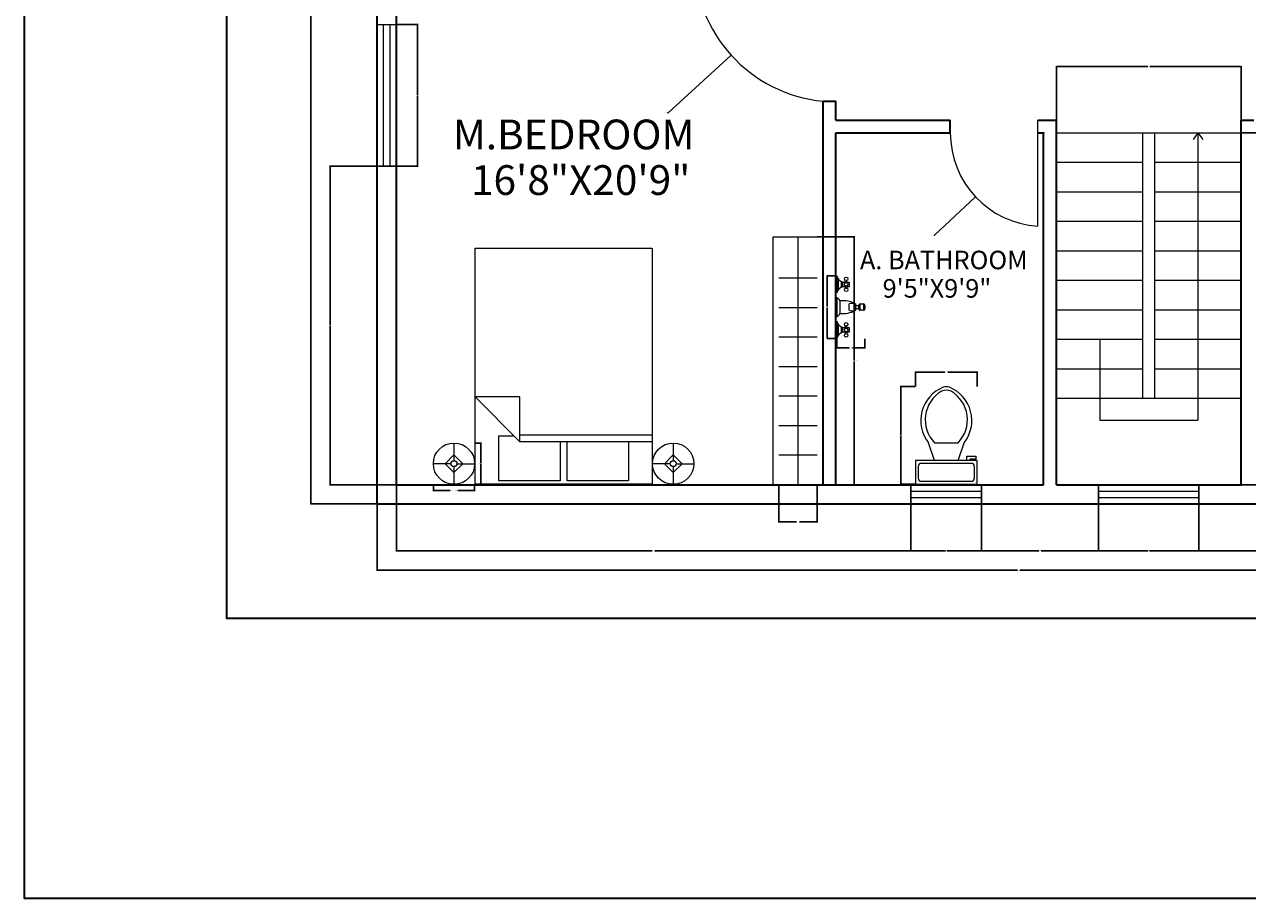
# Model space of a CAD drawing. Units: inches. Extents: x 2286 to 3750, y 1240 to 2345.
# Tile 1 of 7: x 2286 to 2701, y 1240 to 1537. Entities that reach past the tile are written whole.
import ezdxf

# ---------------------------------------------------------------- set-up
doc = ezdxf.new("R2010")
doc.units = ezdxf.units.IN
for name, color, linetype, lineweight in [('A-ANNO-DIMS', 2, 'Continuous', 18), ('A-AREA-IDEN', 7, 'Continuous', 18), ('A-DOOR', 4, 'Continuous', 18), ('A-FLOR-CASE', 8, 'Continuous', 18), ('A-FLOR-FIXT', 9, 'Continuous', 18), ('A-FLOR-STRS', 7, 'Continuous', 18), ('A-FURN', 8, 'Continuous', 18), ('A-GLAZ', 51, 'Continuous', 18), ('A-WALL', 7, 'Continuous', 35)]:
    doc.layers.add(name, color=color, linetype=linetype, lineweight=lineweight)
doc.styles.get("Standard").update_dxf_attribs({"font": 'arial.ttf'})
doc.dimstyles.get("Standard").update_dxf_attribs({"dimtxt": 0.18, "dimasz": 0.18, "dimexe": 0.18, "dimexo": 0.0625, "dimgap": 0.09, "dimtad": 0, "dimtih": 1, "dimtoh": 1, "dimdec": 4, "dimzin": 0, "dimdsep": 46, "dimtxsty": 'Standard', "dimcen": 0.09, "dimadec": 0, "dimazin": 0, "dimtfac": 1, "dimtdec": 4, "dimtofl": 0, "dimtmove": 0, "dimatfit": 3, "dimfxl": 1, "dimtolj": 1, "dimtzin": 0, "dimarcsym": 0})

# ---------------------------------------------------------------- blocks, each defined once
blk = doc.blocks.new('Faucet - Bathroom front')
for p, q in [((-0.5, 4.25), (0.5, 4.25)), ((0.5, 3.75), (-0.5, 3.75)), ((-0.5, 3), (0.5, 3)), ((0.5, 2), (-0.5, 2)), ((-0.25, 3), (-0.25, 3.5)), ((0.25, 3.5), (0.25, 3)), ((-5, 0), (-2.25, 0)), ((-4.5087, 0.25), (-2.7408, 0.25)), ((-4, 1.625), (-4.25, 1.625)), ((-4, 1.375), (-4.25, 1.375)), ((-3.1442, 0.75), (-4.0979, 0.75)), ((-3.25, 1.625), (-3, 1.625)), ((-3.25, 1.375), (-3, 1.375)), ((-1.5, 0), (1.5, 0)), ((-1, 0.5), (1, 0.5)), ((2.25, 0), (5, 0)), ((2.7413, 0.25), (4.5092, 0.25)), ((3.25, 1.625), (3, 1.625)), ((3.25, 1.375), (3, 1.375)), ((4.1058, 0.75), (3.1521, 0.75)), ((4, 1.625), (4.25, 1.625)), ((4, 1.375), (4.25, 1.375))]:
    blk.add_line(p, q)
for points in [[(-0.5, 3.75), (-0.5, 4.25)], [(-0.25, 4.5), (0.25, 4.5)], [(0.5, 4.25), (0.5, 3.75)], [(0.25, 3.5), (-0.25, 3.5)]]:
    blk.add_lwpolyline(points)
for points in [[(-4, 1), (-4, 2), (-3.25, 2), (-3.25, 1)], [(3.25, 1), (3.25, 2), (4, 2), (4, 1)]]:
    blk.add_lwpolyline(points, close=True)
for centre in [(-4.5, 1.5), (-3.625, 1.5), (-2.75, 1.5), (2.75, 1.5), (3.625, 1.5), (4.5, 1.5)]:
    blk.add_circle(centre, 0.2795)
for centre, radius, start, end in [((-0.2575, 4.2575), 0.2426, 88.22243, 181.7776), ((0.2575, 4.2575), 0.2426, 358.2224, 91.77757), ((3, 1), 4.0311, 150.2551, 187.125), ((0.6413, 2.5), 1.246, 156.3417, 203.6583), ((-0.2575, 3.7425), 0.2426, 178.2224, 271.7776), ((0.2575, 3.7425), 0.2426, 268.2224, 1.777565), ((-3, 1), 4.0311, 352.875, 29.74488), ((-0.6413, 2.5), 1.246, 336.3417, 23.65835), ((-5.375, 1.375), 1.4252, 285.2551, 344.7449), ((-1.875, 1.375), 1.4252, 195.2551, 254.7449), ((-0.7962, -0.2038), 0.7327, 106.1502, 163.8498), ((0.7962, -0.2038), 0.7327, 16.1502, 73.84979), ((1.875, 1.375), 1.4252, 285.2551, 344.7449), ((5.375, 1.375), 1.4252, 195.2551, 254.7449)]:
    blk.add_arc(centre, radius, start, end)
blk = doc.blocks.new('Bed - Queen')
for p, q in [((0, -80.00003), (0, 0)), ((0, 0), (59.99999, 0)), ((59.99999, 0), (59.99999, -80.00003)), ((7.99999, -1.2), (28.79998, -1.2)), ((7.99999, -14.4), (7.99999, -1.2)), ((28.79998, -1.2), (28.79998, -14.4)), ((31.19999, -1.2), (51.99999, -1.2)), ((31.19999, -14.4), (31.19999, -1.2)), ((51.99999, -1.2), (51.99999, -16.4)), ((0, -14.4), (44.8, -14.4)), ((59.99999, -29.6), (44.8, -14.4)), ((44.8, -14.4), (44.8, -29.6)), ((51.99999, -16.4), (46.79936, -16.4)), ((44.8, -16.8), (0, -16.8)), ((44.8, -29.6), (59.99999, -29.6)), ((59.99999, -80.00003), (0, -80.00003))]:
    blk.add_line(p, q)
blk = doc.blocks.new('Lamp - Table')
for p, q in [((0, 7), (0, 1)), ((-1, 0), (-7, 0)), ((0, 3), (-3, 0)), ((-3, 0), (0, -3)), ((3, 0), (0, 3)), ((0, -3), (3, 0)), ((1, 0), (7, 0)), ((0, -1), (0, -7))]:
    blk.add_line(p, q)
for radius in [7, 1]:
    blk.add_circle((0, 0), radius)
blk = doc.blocks.new('Toilet - top')
for p, q in [((9.5, -6), (9.5, -2)), ((-8, -8.5), (-8, -8)), ((-7, -8), (-7, -9.5)), ((-4, -8), (-6, -14)), ((4, -8), (6, -14)), ((-10, -8.5), (-8, -8.5)), ((-10, -9.5), (-10, -8.5)), ((-7, -9.5), (-10, -9.5)), ((4, -14), (-4, -14))]:
    blk.add_line(p, q)
blk.add_lwpolyline([(10.5, -8), (10.5, 0), (-10.5, 0), (-10.5, -8)], close=True)
for points in [[(-9.5, -2), (-9.5, -6)], [(8.5, -1), (-8.5, -1)], [(-8.5, -7), (8.5, -7)]]:
    blk.add_lwpolyline(points)
for centre, radius, start, end in [((-8.62, -1.88), 0.884, 81.8699, 188.1301), ((8.62, -1.88), 0.884, 351.8699, 98.1301), ((-8.62, -6.12), 0.884, 171.8699, 278.1301), ((8.62, -6.12), 0.884, 261.8699, 8.1301), ((3.52, -21.58), 12.17, 141.4691, 247.9714), ((4.2, -21.82), 11.33, 136.3677, 238.9468), ((-3.52, -21.58), 12.17, 292.0284, 38.5307), ((-4.2, -21.82), 11.33, 301.053, 43.6321), ((0, -27.88), 4, 245.7318, 294.2682), ((0, -29), 4, 254.8605, 285.1395)]:
    blk.add_arc(centre, radius, start, end)
blk = doc.blocks.new('WIN-48x6p5')
for p, q in [((0, 6.51), (0, 0)), ((0, 4.35), (48, 4.35)), ((48, 6.51), (48, 0)), ((0, 2.16), (48, 2.16))]:
    blk.add_line(p, q)
blk = doc.blocks.new('CLOSET-RAIL-84')
for p, q in [((6.5, 0), (6.5, 84)), ((0, 74), (13, 74)), ((0, 64), (13, 64)), ((0, 54), (13, 54)), ((0, 44), (13, 44)), ((0, 34), (13, 34)), ((0, 24), (13, 24)), ((0, 14), (13, 14))]:
    blk.add_line(p, q)
blk = doc.blocks.new('*D24')
at = {"layer": 'A-ANNO-DIMS', "color": 0, "lineweight": -2, "transparency": 16777216}
for p, q in [((2424.82, 1380.78), (2424.82, 1378.56)), ((2438.82, 1380.78), (2438.82, 1378.56)), ((2425, 1378.74), (2430.48, 1378.74)), ((2438.64, 1378.74), (2433.16, 1378.74))]:
    blk.add_line(p, q, dxfattribs=at)
at = {"layer": 'A-ANNO-DIMS', "color": 0, "transparency": 16777216}
for points in [[(2425, 1378.77), (2425, 1378.71), (2424.82, 1378.74)], [(2438.64, 1378.77), (2438.64, 1378.71), (2438.82, 1378.74)]]:
    blk.add_solid(points, dxfattribs=at)
at = {"layer": 'Defpoints', "color": 0, "transparency": 16777216}
for p in [(2424.82, 1380.84), (2438.82, 1380.84), (2438.82, 1378.74)]:
    blk.add_point(p, dxfattribs=at)
at = {"layer": 'A-ANNO-DIMS', "color": 0, "transparency": 16777216, "insert": (2431.82, 1378.74), "char_height": 0.18, "attachment_point": 5}
blk.add_mtext('\\A1;TABLE LAMP 14 TYP.', dxfattribs=at)
blk = doc.blocks.new('*D25')
at = {"layer": 'A-ANNO-DIMS', "color": 0, "lineweight": -2, "transparency": 16777216}
for p, q in [((2438.88, 1394.84), (2441.1, 1394.84)), ((2440.92, 1394.66), (2440.92, 1388.02)), ((2440.92, 1381.02), (2440.92, 1387.66)), ((2438.88, 1380.84), (2441.1, 1380.84))]:
    blk.add_line(p, q, dxfattribs=at)
at = {"layer": 'A-ANNO-DIMS', "color": 0, "transparency": 16777216}
for points in [[(2440.89, 1394.66), (2440.95, 1394.66), (2440.92, 1394.84)], [(2440.89, 1381.02), (2440.95, 1381.02), (2440.92, 1380.84)]]:
    blk.add_solid(points, dxfattribs=at)
at = {"layer": 'Defpoints', "color": 0, "transparency": 16777216}
for p in [(2438.82, 1394.84), (2440.92, 1394.84), (2438.82, 1380.84)]:
    blk.add_point(p, dxfattribs=at)
at = {"layer": 'A-ANNO-DIMS', "color": 0, "transparency": 16777216, "insert": (2440.92, 1387.84), "char_height": 0.18, "attachment_point": 5}
blk.add_mtext('\\A1;14 TYP.', dxfattribs=at)
blk = doc.blocks.new('*D30')
at = {"layer": 'A-ANNO-DIMS', "color": 0, "lineweight": -2, "transparency": 16777216}
for p, q in [((2588.15, 1413.95), (2583.07, 1413.95)), ((2583.25, 1413.77), (2583.25, 1397.61)), ((2583.25, 1381.08), (2583.25, 1397.24)), ((2588.15, 1380.9), (2583.07, 1380.9))]:
    blk.add_line(p, q, dxfattribs=at)
at = {"layer": 'A-ANNO-DIMS', "color": 0, "transparency": 16777216}
for points in [[(2583.22, 1413.77), (2583.28, 1413.77), (2583.25, 1413.95)], [(2583.22, 1381.08), (2583.28, 1381.08), (2583.25, 1380.9)]]:
    blk.add_solid(points, dxfattribs=at)
at = {"layer": 'Defpoints', "color": 0, "transparency": 16777216}
for p in [(2588.21, 1413.95), (2583.25, 1380.9), (2588.21, 1380.9)]:
    blk.add_point(p, dxfattribs=at)
at = {"layer": 'A-ANNO-DIMS', "color": 0, "transparency": 16777216, "insert": (2583.25, 1397.42), "char_height": 0.18, "attachment_point": 5}
blk.add_mtext('\\A1;WC 33 TYP.', dxfattribs=at)
blk = doc.blocks.new('*D31')
at = {"layer": 'A-ANNO-DIMS', "color": 0, "lineweight": -2, "transparency": 16777216}
for p, q in [((2588.21, 1414.01), (2588.21, 1419.08)), ((2588.39, 1418.9), (2598.18, 1418.9)), ((2609.03, 1418.9), (2599.24, 1418.9)), ((2609.21, 1414.01), (2609.21, 1419.08))]:
    blk.add_line(p, q, dxfattribs=at)
at = {"layer": 'A-ANNO-DIMS', "color": 0, "transparency": 16777216}
for points in [[(2588.39, 1418.93), (2588.39, 1418.87), (2588.21, 1418.9)], [(2609.03, 1418.93), (2609.03, 1418.87), (2609.21, 1418.9)]]:
    blk.add_solid(points, dxfattribs=at)
at = {"layer": 'Defpoints', "color": 0, "transparency": 16777216}
for p in [(2588.21, 1418.9), (2588.21, 1413.95), (2609.21, 1413.95)]:
    blk.add_point(p, dxfattribs=at)
at = {"layer": 'A-ANNO-DIMS', "color": 0, "transparency": 16777216, "insert": (2598.71, 1418.9), "char_height": 0.18, "attachment_point": 5}
blk.add_mtext('\\A1;21 TYP.', dxfattribs=at)
blk = doc.blocks.new('*D36')
at = {"layer": 'A-ANNO-DIMS', "color": 0, "lineweight": -2, "transparency": 16777216}
for p, q in [((2412.36, 1536.75), (2419.68, 1536.75)), ((2419.5, 1536.57), (2419.5, 1512.93)), ((2419.5, 1488.93), (2419.5, 1512.56)), ((2412.36, 1488.75), (2419.68, 1488.75))]:
    blk.add_line(p, q, dxfattribs=at)
at = {"layer": 'A-ANNO-DIMS', "color": 0, "transparency": 16777216}
for points in [[(2419.47, 1536.57), (2419.53, 1536.57), (2419.5, 1536.75)], [(2419.47, 1488.93), (2419.53, 1488.93), (2419.5, 1488.75)]]:
    blk.add_solid(points, dxfattribs=at)
at = {"layer": 'Defpoints', "color": 0, "transparency": 16777216}
for p in [(2412.3, 1536.75), (2419.5, 1536.75), (2412.3, 1488.75)]:
    blk.add_point(p, dxfattribs=at)
at = {"layer": 'A-ANNO-DIMS', "color": 0, "transparency": 16777216, "insert": (2419.5, 1512.75), "char_height": 0.18, "attachment_point": 5}
blk.add_mtext('\\A1;WINDOW 48 TYP.', dxfattribs=at)
blk = doc.blocks.new('*D37')
at = {"layer": 'A-ANNO-DIMS', "color": 0, "lineweight": -2, "transparency": 16777216}
for p, q in [((2405.79, 1536.81), (2405.79, 1544.13)), ((2405.97, 1543.95), (2408.59, 1543.95)), ((2412.12, 1543.95), (2409.5, 1543.95)), ((2412.3, 1536.81), (2412.3, 1544.13))]:
    blk.add_line(p, q, dxfattribs=at)
at = {"layer": 'A-ANNO-DIMS', "color": 0, "transparency": 16777216}
for points in [[(2405.97, 1543.98), (2405.97, 1543.92), (2405.79, 1543.95)], [(2412.12, 1543.98), (2412.12, 1543.92), (2412.3, 1543.95)]]:
    blk.add_solid(points, dxfattribs=at)
at = {"layer": 'Defpoints', "color": 0, "transparency": 16777216}
for p in [(2405.79, 1543.95), (2405.79, 1536.75), (2412.3, 1536.75)]:
    blk.add_point(p, dxfattribs=at)
at = {"layer": 'A-ANNO-DIMS', "color": 0, "transparency": 16777216, "insert": (2409.04, 1543.95), "char_height": 0.18, "attachment_point": 5}
blk.add_mtext('\\A1;7 TYP.', dxfattribs=at)
blk = doc.blocks.new('*D38')
at = {"layer": 'A-ANNO-DIMS', "color": 0, "lineweight": -2, "transparency": 16777216}
for p, q in [((2554.98, 1464.69), (2567.7, 1464.69)), ((2567.52, 1464.51), (2567.52, 1422.87)), ((2567.52, 1380.87), (2567.52, 1422.51)), ((2554.98, 1380.69), (2567.7, 1380.69))]:
    blk.add_line(p, q, dxfattribs=at)
at = {"layer": 'A-ANNO-DIMS', "color": 0, "transparency": 16777216}
for points in [[(2567.49, 1464.51), (2567.55, 1464.51), (2567.52, 1464.69)], [(2567.49, 1380.87), (2567.55, 1380.87), (2567.52, 1380.69)]]:
    blk.add_solid(points, dxfattribs=at)
at = {"layer": 'Defpoints', "color": 0, "transparency": 16777216}
for p in [(2554.92, 1464.69), (2554.92, 1380.69), (2567.52, 1380.69)]:
    blk.add_point(p, dxfattribs=at)
at = {"layer": 'A-ANNO-DIMS', "color": 0, "transparency": 16777216, "insert": (2567.52, 1422.69), "char_height": 0.18, "attachment_point": 5}
blk.add_mtext('\\A1;CLOSET RAIL 84 TYP.', dxfattribs=at)
blk = doc.blocks.new('*D39')
at = {"layer": 'A-ANNO-DIMS', "color": 0, "lineweight": -2, "transparency": 16777216}
for p, q in [((2541.92, 1380.63), (2541.92, 1367.91)), ((2554.92, 1380.63), (2554.92, 1367.91)), ((2542.1, 1368.09), (2547.9, 1368.09)), ((2554.74, 1368.09), (2548.94, 1368.09))]:
    blk.add_line(p, q, dxfattribs=at)
at = {"layer": 'A-ANNO-DIMS', "color": 0, "transparency": 16777216}
for points in [[(2542.1, 1368.12), (2542.1, 1368.06), (2541.92, 1368.09)], [(2554.74, 1368.12), (2554.74, 1368.06), (2554.92, 1368.09)]]:
    blk.add_solid(points, dxfattribs=at)
at = {"layer": 'Defpoints', "color": 0, "transparency": 16777216}
for p in [(2541.92, 1380.69), (2554.92, 1380.69), (2541.92, 1368.09)]:
    blk.add_point(p, dxfattribs=at)
at = {"layer": 'A-ANNO-DIMS', "color": 0, "transparency": 16777216, "insert": (2548.42, 1368.09), "char_height": 0.18, "attachment_point": 5}
blk.add_mtext('\\A1;13 TYP.', dxfattribs=at)
blk = doc.blocks.new('*D40')
at = {"layer": 'A-ANNO-DIMS', "color": 0, "lineweight": -2, "transparency": 16777216}
for p, q in [((2561.48, 1451.56), (2558.17, 1451.56)), ((2558.35, 1451.38), (2558.35, 1441.09)), ((2558.35, 1430.44), (2558.35, 1440.73)), ((2561.48, 1430.26), (2558.17, 1430.26))]:
    blk.add_line(p, q, dxfattribs=at)
at = {"layer": 'A-ANNO-DIMS', "color": 0, "transparency": 16777216}
for points in [[(2558.32, 1451.38), (2558.38, 1451.38), (2558.35, 1451.56)], [(2558.32, 1430.44), (2558.38, 1430.44), (2558.35, 1430.26)]]:
    blk.add_solid(points, dxfattribs=at)
at = {"layer": 'Defpoints', "color": 0, "transparency": 16777216}
for p in [(2561.55, 1451.56), (2558.35, 1430.26), (2561.55, 1430.26)]:
    blk.add_point(p, dxfattribs=at)
at = {"layer": 'A-ANNO-DIMS', "color": 0, "transparency": 16777216, "insert": (2558.35, 1440.91), "char_height": 0.18, "attachment_point": 5}
blk.add_mtext('\\A1;BATH TAP 21 TYP.', dxfattribs=at)
blk = doc.blocks.new('*D41')
at = {"layer": 'A-ANNO-DIMS', "color": 0, "lineweight": -2, "transparency": 16777216}
for p, q in [((2561.55, 1430.2), (2561.55, 1426.88)), ((2561.73, 1427.06), (2565.82, 1427.06)), ((2570.96, 1427.06), (2566.86, 1427.06)), ((2571.14, 1430.2), (2571.14, 1426.88))]:
    blk.add_line(p, q, dxfattribs=at)
at = {"layer": 'A-ANNO-DIMS', "color": 0, "transparency": 16777216}
for points in [[(2561.73, 1427.09), (2561.73, 1427.03), (2561.55, 1427.06)], [(2570.96, 1427.09), (2570.96, 1427.03), (2571.14, 1427.06)]]:
    blk.add_solid(points, dxfattribs=at)
at = {"layer": 'Defpoints', "color": 0, "transparency": 16777216}
for p in [(2561.55, 1430.26), (2571.14, 1430.26), (2571.14, 1427.06)]:
    blk.add_point(p, dxfattribs=at)
at = {"layer": 'A-ANNO-DIMS', "color": 0, "transparency": 16777216, "insert": (2566.34, 1427.06), "char_height": 0.18, "attachment_point": 5}
blk.add_mtext('\\A1;10 TYP.', dxfattribs=at)
blk = doc.blocks.new('*D74')
at = {"layer": 'A-ANNO-DIMS', "color": 0, "lineweight": -2, "transparency": 16777216}
for p, q in [((2405.79, 1374.12), (2405.79, 1351.55)), ((2840.66, 1374.12), (2840.66, 1351.55)), ((2405.97, 1351.73), (2622.83, 1351.73)), ((2840.48, 1351.73), (2623.62, 1351.73))]:
    blk.add_line(p, q, dxfattribs=at)
at = {"layer": 'A-ANNO-DIMS', "color": 0, "transparency": 16777216}
for points in [[(2405.97, 1351.76), (2405.97, 1351.7), (2405.79, 1351.73)], [(2840.48, 1351.76), (2840.48, 1351.7), (2840.66, 1351.73)]]:
    blk.add_solid(points, dxfattribs=at)
at = {"layer": 'Defpoints', "color": 0, "transparency": 16777216}
for p in [(2405.79, 1374.18), (2840.66, 1374.18), (2840.66, 1351.73)]:
    blk.add_point(p, dxfattribs=at)
at = {"layer": 'A-ANNO-DIMS', "color": 0, "transparency": 16777216, "insert": (2623.23, 1351.73), "char_height": 0.18, "attachment_point": 5}
blk.add_mtext('\\A1;434.9', dxfattribs=at)
blk = doc.blocks.new('*D75')
at = {"layer": 'A-ANNO-DIMS', "color": 0, "lineweight": -2, "transparency": 16777216}
for p, q in [((2405.73, 1741.53), (2383.16, 1741.53)), ((2383.34, 1741.35), (2383.34, 1558.04)), ((2383.34, 1374.36), (2383.34, 1557.67)), ((2405.73, 1374.18), (2383.16, 1374.18))]:
    blk.add_line(p, q, dxfattribs=at)
at = {"layer": 'A-ANNO-DIMS', "color": 0, "transparency": 16777216}
for points in [[(2383.31, 1741.35), (2383.37, 1741.35), (2383.34, 1741.53)], [(2383.31, 1374.36), (2383.37, 1374.36), (2383.34, 1374.18)]]:
    blk.add_solid(points, dxfattribs=at)
at = {"layer": 'Defpoints', "color": 0, "transparency": 16777216}
for p in [(2383.34, 1741.53), (2405.79, 1741.53), (2405.79, 1374.18)]:
    blk.add_point(p, dxfattribs=at)
at = {"layer": 'A-ANNO-DIMS', "color": 0, "transparency": 16777216, "insert": (2383.34, 1557.85), "char_height": 0.18, "attachment_point": 5}
blk.add_mtext('\\A1;367.35', dxfattribs=at)
blk = doc.blocks.new('*D80')
at = {"layer": 'A-ANNO-DIMS', "color": 0, "lineweight": -2, "transparency": 16777216}
for p, q in [((2636.05, 1500.07), (2636.05, 1522.63)), ((2636.23, 1522.45), (2667.03, 1522.45)), ((2698.47, 1522.45), (2667.68, 1522.45)), ((2698.65, 1500.07), (2698.65, 1522.63))]:
    blk.add_line(p, q, dxfattribs=at)
at = {"layer": 'A-ANNO-DIMS', "color": 0, "transparency": 16777216}
for points in [[(2636.23, 1522.48), (2636.23, 1522.42), (2636.05, 1522.45)], [(2698.47, 1522.48), (2698.47, 1522.42), (2698.65, 1522.45)]]:
    blk.add_solid(points, dxfattribs=at)
at = {"layer": 'Defpoints', "color": 0, "transparency": 16777216}
for p in [(2698.65, 1522.45), (2636.05, 1500), (2698.65, 1500)]:
    blk.add_point(p, dxfattribs=at)
at = {"layer": 'A-ANNO-DIMS', "color": 0, "transparency": 16777216, "insert": (2667.35, 1522.45), "char_height": 0.18, "attachment_point": 5}
blk.add_mtext('\\A1;62.6', dxfattribs=at)
blk = doc.blocks.new('*D81')
at = {"layer": 'A-ANNO-DIMS', "color": 0, "lineweight": -2, "transparency": 16777216}
for p, q in [((2698.72, 1500), (2721.28, 1500)), ((2721.1, 1499.82), (2721.1, 1440.53)), ((2721.1, 1380.87), (2721.1, 1440.16)), ((2698.72, 1380.69), (2721.28, 1380.69))]:
    blk.add_line(p, q, dxfattribs=at)
at = {"layer": 'A-ANNO-DIMS', "color": 0, "transparency": 16777216}
for points in [[(2721.07, 1499.82), (2721.13, 1499.82), (2721.1, 1500)], [(2721.07, 1380.87), (2721.13, 1380.87), (2721.1, 1380.69)]]:
    blk.add_solid(points, dxfattribs=at)
at = {"layer": 'Defpoints', "color": 0, "transparency": 16777216}
for p in [(2698.65, 1500), (2698.65, 1380.69), (2721.1, 1380.69)]:
    blk.add_point(p, dxfattribs=at)
at = {"layer": 'A-ANNO-DIMS', "color": 0, "transparency": 16777216, "insert": (2721.1, 1440.35), "char_height": 0.18, "attachment_point": 5}
blk.add_mtext('\\A1;119.32', dxfattribs=at)
blk = doc.blocks.new('*D82')
at = {"layer": 'A-ANNO-DIMS', "color": 0, "lineweight": -2, "transparency": 16777216}
for p, q in [((2412.23, 1488.75), (2389.67, 1488.75)), ((2389.85, 1488.57), (2389.85, 1434.9)), ((2389.85, 1380.87), (2389.85, 1434.54)), ((2412.23, 1380.69), (2389.67, 1380.69))]:
    blk.add_line(p, q, dxfattribs=at)
at = {"layer": 'A-ANNO-DIMS', "color": 0, "transparency": 16777216}
for points in [[(2389.82, 1488.57), (2389.88, 1488.57), (2389.85, 1488.75)], [(2389.82, 1380.87), (2389.88, 1380.87), (2389.85, 1380.69)]]:
    blk.add_solid(points, dxfattribs=at)
at = {"layer": 'Defpoints', "color": 0, "transparency": 16777216}
for p in [(2389.85, 1488.75), (2412.3, 1488.75), (2412.3, 1380.69)]:
    blk.add_point(p, dxfattribs=at)
at = {"layer": 'A-ANNO-DIMS', "color": 0, "transparency": 16777216, "insert": (2389.85, 1434.72), "char_height": 0.18, "attachment_point": 5}
blk.add_mtext('\\A1;108.06', dxfattribs=at)
blk = doc.blocks.new('*D87')
at = {"layer": 'A-ANNO-DIMS', "color": 0, "lineweight": -2, "transparency": 16777216}
for p, q in [((2586.64, 1380.63), (2586.64, 1358.06)), ((2610.64, 1380.63), (2610.64, 1358.06)), ((2586.82, 1358.24), (2598.42, 1358.24)), ((2610.46, 1358.24), (2598.86, 1358.24))]:
    blk.add_line(p, q, dxfattribs=at)
at = {"layer": 'A-ANNO-DIMS', "color": 0, "transparency": 16777216}
for points in [[(2586.82, 1358.27), (2586.82, 1358.21), (2586.64, 1358.24)], [(2610.46, 1358.27), (2610.46, 1358.21), (2610.64, 1358.24)]]:
    blk.add_solid(points, dxfattribs=at)
at = {"layer": 'Defpoints', "color": 0, "transparency": 16777216}
for p in [(2586.64, 1380.69), (2610.64, 1380.69), (2586.64, 1358.24)]:
    blk.add_point(p, dxfattribs=at)
at = {"layer": 'A-ANNO-DIMS', "color": 0, "transparency": 16777216, "insert": (2598.64, 1358.24), "char_height": 0.18, "attachment_point": 5}
blk.add_mtext('\\A1;24', dxfattribs=at)
blk = doc.blocks.new('*D88')
at = {"layer": 'A-ANNO-DIMS', "color": 0, "lineweight": -2, "transparency": 16777216}
for p, q in [((2610.64, 1380.63), (2610.64, 1358.06)), ((2650.35, 1380.63), (2650.35, 1358.06)), ((2610.82, 1358.24), (2630.12, 1358.24)), ((2650.17, 1358.24), (2630.87, 1358.24))]:
    blk.add_line(p, q, dxfattribs=at)
at = {"layer": 'A-ANNO-DIMS', "color": 0, "transparency": 16777216}
for points in [[(2610.82, 1358.27), (2610.82, 1358.21), (2610.64, 1358.24)], [(2650.17, 1358.27), (2650.17, 1358.21), (2650.35, 1358.24)]]:
    blk.add_solid(points, dxfattribs=at)
at = {"layer": 'Defpoints', "color": 0, "transparency": 16777216}
for p in [(2610.64, 1380.69), (2650.35, 1380.69), (2610.64, 1358.24)]:
    blk.add_point(p, dxfattribs=at)
at = {"layer": 'A-ANNO-DIMS', "color": 0, "transparency": 16777216, "insert": (2630.5, 1358.24), "char_height": 0.18, "attachment_point": 5}
blk.add_mtext('\\A1;39.71', dxfattribs=at)
blk = doc.blocks.new('*D89')
at = {"layer": 'A-ANNO-DIMS', "color": 0, "lineweight": -2, "transparency": 16777216}
for p, q in [((2650.35, 1380.63), (2650.35, 1358.06)), ((2684.35, 1380.63), (2684.35, 1358.06)), ((2650.53, 1358.24), (2667.13, 1358.24)), ((2684.17, 1358.24), (2667.57, 1358.24))]:
    blk.add_line(p, q, dxfattribs=at)
at = {"layer": 'A-ANNO-DIMS', "color": 0, "transparency": 16777216}
for points in [[(2650.53, 1358.27), (2650.53, 1358.21), (2650.35, 1358.24)], [(2684.17, 1358.27), (2684.17, 1358.21), (2684.35, 1358.24)]]:
    blk.add_solid(points, dxfattribs=at)
at = {"layer": 'Defpoints', "color": 0, "transparency": 16777216}
for p in [(2650.35, 1380.69), (2684.35, 1380.69), (2650.35, 1358.24)]:
    blk.add_point(p, dxfattribs=at)
at = {"layer": 'A-ANNO-DIMS', "color": 0, "transparency": 16777216, "insert": (2667.35, 1358.24), "char_height": 0.18, "attachment_point": 5}
blk.add_mtext('\\A1;34', dxfattribs=at)
blk = doc.blocks.new('*D90')
at = {"layer": 'A-ANNO-DIMS', "color": 0, "lineweight": -2, "transparency": 16777216}
for p, q in [((2684.35, 1380.63), (2684.35, 1358.06)), ((2731.42, 1380.63), (2731.42, 1358.06)), ((2684.53, 1358.24), (2707.49, 1358.24)), ((2731.24, 1358.24), (2708.28, 1358.24))]:
    blk.add_line(p, q, dxfattribs=at)
at = {"layer": 'A-ANNO-DIMS', "color": 0, "transparency": 16777216}
for points in [[(2684.53, 1358.27), (2684.53, 1358.21), (2684.35, 1358.24)], [(2731.24, 1358.27), (2731.24, 1358.21), (2731.42, 1358.24)]]:
    blk.add_solid(points, dxfattribs=at)
at = {"layer": 'Defpoints', "color": 0, "transparency": 16777216}
for p in [(2684.35, 1380.69), (2731.42, 1380.69), (2684.35, 1358.24)]:
    blk.add_point(p, dxfattribs=at)
at = {"layer": 'A-ANNO-DIMS', "color": 0, "transparency": 16777216, "insert": (2707.88, 1358.24), "char_height": 0.18, "attachment_point": 5}
blk.add_mtext('\\A1;47.07', dxfattribs=at)
blk = doc.blocks.new('*D91')
at = {"layer": 'A-ANNO-DIMS', "color": 0, "lineweight": -2, "transparency": 16777216}
for p, q in [((2412.3, 1380.63), (2412.3, 1358.06)), ((2586.64, 1380.63), (2586.64, 1358.06)), ((2412.48, 1358.24), (2499.01, 1358.24)), ((2586.46, 1358.24), (2499.93, 1358.24))]:
    blk.add_line(p, q, dxfattribs=at)
at = {"layer": 'A-ANNO-DIMS', "color": 0, "transparency": 16777216}
for points in [[(2412.48, 1358.27), (2412.48, 1358.21), (2412.3, 1358.24)], [(2586.46, 1358.27), (2586.46, 1358.21), (2586.64, 1358.24)]]:
    blk.add_solid(points, dxfattribs=at)
at = {"layer": 'Defpoints', "color": 0, "transparency": 16777216}
for p in [(2412.3, 1380.69), (2586.64, 1380.69), (2412.3, 1358.24)]:
    blk.add_point(p, dxfattribs=at)
at = {"layer": 'A-ANNO-DIMS', "color": 0, "transparency": 16777216, "insert": (2499.47, 1358.24), "char_height": 0.18, "attachment_point": 5}
blk.add_mtext('\\A1;174.35', dxfattribs=at)
blk = doc.blocks.new('*D128')
at = {"layer": 'A-ANNO-DIMS', "color": 0, "lineweight": -2, "transparency": 16777216}
for p, q in [((2561.39, 1558.75), (2561.57, 1558.75)), ((2561.48, 1558.66), (2561.48, 1558.84)), ((2504.41, 1506.84), (2525.67, 1526.18)), ((2504.23, 1506.84), (2504.41, 1506.84))]:
    blk.add_line(p, q, dxfattribs=at)
at = {"layer": 'A-ANNO-DIMS', "color": 0, "transparency": 16777216}
blk.add_solid([(2525.65, 1526.2), (2525.69, 1526.16), (2525.81, 1526.3)], dxfattribs=at)
at = {"layer": 'Defpoints', "color": 0, "transparency": 16777216}
for p in [(2561.48, 1558.75), (2525.81, 1526.3)]:
    blk.add_point(p, dxfattribs=at)
at = {"layer": 'A-ANNO-DIMS', "color": 0, "transparency": 16777216, "insert": (2503.75, 1506.84), "char_height": 0.18, "attachment_point": 5}
blk.add_mtext('\\A1;R48.22', dxfattribs=at)
blk = doc.blocks.new('*D131')
at = {"layer": 'A-ANNO-DIMS', "color": 0, "lineweight": -2, "transparency": 16777216}
for p, q in [((2631.69, 1500), (2631.87, 1500)), ((2631.78, 1499.91), (2631.78, 1500.09)), ((2594.73, 1465.3), (2608.49, 1478.19)), ((2594.55, 1465.3), (2594.73, 1465.3))]:
    blk.add_line(p, q, dxfattribs=at)
at = {"layer": 'A-ANNO-DIMS', "color": 0, "transparency": 16777216}
blk.add_solid([(2608.47, 1478.21), (2608.51, 1478.17), (2608.62, 1478.31)], dxfattribs=at)
at = {"layer": 'Defpoints', "color": 0, "transparency": 16777216}
for p in [(2631.78, 1500), (2608.62, 1478.31)]:
    blk.add_point(p, dxfattribs=at)
at = {"layer": 'A-ANNO-DIMS', "color": 0, "transparency": 16777216, "insert": (2594.07, 1465.3), "char_height": 0.18, "attachment_point": 5}
blk.add_mtext('\\A1;R31.73', dxfattribs=at)

msp = doc.modelspace()

# ---------------------------------------------------------------- linework, layer by layer
at = {"layer": 'A-DOOR'}
msp.add_line((2629.7107, 1468.3424), (2629.7107, 1504.3424), dxfattribs=at)
for centre, radius, end in [((2561.4757, 1558.746), 48.2156, 264.579918), ((2631.7781, 1500.0037), 31.7287, 266.263985)]:
    msp.add_arc(centre, radius, 180, end, dxfattribs=at)
at = {"layer": 'A-FLOR-CASE'}
for p, q in [((2556.9214, 1464.6885), (2539.9214, 1464.6885)), ((2539.9214, 1464.6885), (2539.9214, 1380.6885)), ((2556.9214, 1464.6885), (2556.9214, 1380.6885))]:
    msp.add_line(p, q, dxfattribs=at)
at = {"layer": 'A-FLOR-STRS'}
for p, q in [((2636.0494, 1500.0037), (2698.6534, 1500.0037)), ((2665.3514, 1410.0037), (2665.3514, 1500.0037)), ((2669.3514, 1410.0037), (2669.3514, 1500.0037)), ((2684.0024, 1500.0037), (2682.3704, 1497.7855)), ((2684.0024, 1500.0037), (2684.0024, 1402.5732)), ((2684.0024, 1500.0037), (2685.6344, 1497.7855)), ((2636.0494, 1490.0037), (2665.3514, 1490.0037)), ((2669.3514, 1490.0037), (2698.6534, 1490.0037)), ((2636.0494, 1480.0037), (2665.3514, 1480.0037)), ((2669.3514, 1480.0037), (2698.6534, 1480.0037)), ((2636.0494, 1470.0037), (2665.3514, 1470.0037)), ((2669.3514, 1470.0037), (2698.6534, 1470.0037)), ((2636.0494, 1460.0037), (2665.3514, 1460.0037)), ((2669.3514, 1460.0037), (2698.6534, 1460.0037)), ((2636.0494, 1450.0037), (2665.3514, 1450.0037)), ((2669.3514, 1450.0037), (2698.6534, 1450.0037)), ((2636.0494, 1440.0037), (2665.3514, 1440.0037)), ((2669.3514, 1440.0037), (2698.6534, 1440.0037)), ((2636.0494, 1430.0037), (2665.3514, 1430.0037)), ((2650.7004, 1430.0037), (2650.7004, 1402.5732)), ((2669.3514, 1430.0037), (2698.6534, 1430.0037)), ((2636.0494, 1420.0037), (2665.3514, 1420.0037)), ((2669.3514, 1420.0037), (2698.6534, 1420.0037)), ((2636.0494, 1410.0037), (2698.6534, 1410.0037)), ((2650.7004, 1402.5732), (2684.0024, 1402.5732))]:
    msp.add_line(p, q, dxfattribs=at)
at = {"layer": 'A-GLAZ'}
for p, q in [((2586.642, 1374.1804), (2586.642, 1380.6885)), ((2610.642, 1374.1804), (2610.642, 1380.6885)), ((2650.3514, 1380.6885), (2650.3514, 1374.1804)), ((2650.3514, 1380.6885), (2650.3514, 1374.1804)), ((2684.3514, 1380.6885), (2684.3514, 1374.1804)), ((2586.642, 1378.5285), (2610.642, 1378.5285)), ((2650.3514, 1378.5285), (2684.3514, 1378.5285)), ((2586.642, 1376.3404), (2610.642, 1376.3404)), ((2650.3514, 1376.3404), (2684.3514, 1376.3404))]:
    msp.add_line(p, q, dxfattribs=at)
at = {"layer": 'A-WALL'}
for p, q in [((2405.7888, 1374.1804), (2405.7888, 1741.5266)), ((2412.2969, 1380.6885), (2412.2969, 1735.0185)), ((2556.9214, 1380.6885), (2556.9214, 1510.746)), ((2556.9214, 1510.746), (2561.2601, 1510.746)), ((2561.2601, 1504.3424), (2561.2601, 1510.746)), ((2561.2601, 1504.3424), (2600.0494, 1504.3424)), ((2600.0494, 1500.0037), (2600.0494, 1504.3424)), ((2629.7107, 1504.3424), (2636.0494, 1504.3424)), ((2636.0494, 1380.6885), (2636.0494, 1504.3424)), ((2698.6534, 1380.6885), (2698.6534, 1504.3424)), ((2698.6534, 1504.3424), (2702.9921, 1504.3424)), ((2561.2601, 1380.6885), (2561.2601, 1500.0037)), ((2561.2601, 1500.0037), (2600.0494, 1500.0037)), ((2629.7107, 1500.0037), (2631.7107, 1500.0037)), ((2631.7107, 1380.6885), (2631.7107, 1500.0037)), ((2412.2969, 1380.6885), (2631.7107, 1380.6885)), ((2636.0494, 1380.6885), (2698.6534, 1380.6885)), ((2405.7888, 1374.1804), (2840.6637, 1374.1804))]:
    msp.add_line(p, q, dxfattribs=at)
for points in [[(2286.2079, 2344.8717), (3750.2574, 2344.8717), (3750.2574, 1240.4105), (2286.2079, 1240.4105)], [(2354.794, 2286.8809), (3673.7575, 2286.8809), (3673.7575, 1335.3046), (2354.794, 1335.3046)]]:
    msp.add_lwpolyline(points, close=True, dxfattribs=at)

# ---------------------------------------------------------------- block references
at = {"layer": 'A-FLOR-CASE', "rotation": 180}
msp.add_blockref('CLOSET-RAIL-84', (2554.9214, 1464.6885), dxfattribs=at)
at = {"layer": 'A-FLOR-FIXT', "xscale": 2.130333955726564, "yscale": 2.130333955726564, "zscale": 2.130333955726564, "rotation": 270}
msp.add_blockref('Faucet - Bathroom front', (2561.5463, 1440.9113), dxfattribs=at)
at = {"layer": 'A-FLOR-FIXT', "rotation": 180}
msp.add_blockref('Toilet - top', (2598.7118, 1380.8997), dxfattribs=at)
at = {"layer": 'A-FURN', "rotation": 180}
msp.add_blockref('Bed - Queen', (2498.9812, 1380.8751), dxfattribs=at)
at = {"layer": 'A-FURN'}
for p in [(2431.8167, 1387.8428), (2506.1325, 1387.8428)]:
    msp.add_blockref('Lamp - Table', p, dxfattribs=at)
at = {"layer": 'A-GLAZ', "rotation": 89.99999999999736}
msp.add_blockref('WIN-48x6p5', (2412.2969, 1488.746), dxfattribs=at)

# ---------------------------------------------------------------- texts
at = {"layer": 'A-AREA-IDEN'}
for s, height, p in [('M.BEDROOM', 10.08366, (2431.4138, 1494.408)), ('  16\'8"X20\'9"', 10.083661, (2431.4138, 1478.9537)), ('A. BATHROOM', 6.282441, (2569.4371, 1453.754)), ('    9\'5"X9\'9"', 6.282441, (2569.4371, 1444.1255))]:
    msp.add_text(s, height=height, dxfattribs=at).set_placement(p)

# ---------------------------------------------------------------- dimensions: what is measured, and where the dimension line sits
at = {"layer": 'A-ANNO-DIMS'}
for base, p1, p2, angle, override, picture, middle in [((2383.3388, 1741.5266), (2405.7888, 1374.1804), (2405.7888, 1741.5266), 90, {"dimdec": 2, "dimlfac": 1, "dimrnd": 0, "dimzin": 0, "dimdsep": 46, "dimlunit": 2}, '*D75', (2383.3388, 1557.8535)), ((2721.1034, 1380.6885), (2698.6534, 1500.0037), (2698.6534, 1380.6885), 270, {"dimdec": 2, "dimlfac": 1, "dimrnd": 0, "dimzin": 0, "dimdsep": 46, "dimlunit": 2}, '*D81', (2721.1034, 1440.3461)), ((2389.8469, 1488.746), (2412.2969, 1380.6885), (2412.2969, 1488.746), 90, {"dimdec": 2, "dimlfac": 1, "dimrnd": 0, "dimzin": 0, "dimdsep": 46, "dimlunit": 2}, '*D82', (2389.8469, 1434.7172)), ((2412.2969, 1358.2385), (2586.642, 1380.6885), (2412.2969, 1380.6885), 180, {"dimdec": 2, "dimlfac": 1, "dimrnd": 0, "dimzin": 0, "dimdsep": 46, "dimlunit": 2}, '*D91', (2499.4694, 1358.2385)), ((2586.642, 1358.2385), (2610.642, 1380.6885), (2586.642, 1380.6885), 180, {"dimdec": 0, "dimlfac": 1, "dimrnd": 0, "dimzin": 0, "dimdsep": 46, "dimlunit": 2}, '*D87', (2598.642, 1358.2385)), ((2610.642, 1358.2385), (2650.3514, 1380.6885), (2610.642, 1380.6885), 180, {"dimdec": 2, "dimlfac": 1, "dimrnd": 0, "dimzin": 0, "dimdsep": 46, "dimlunit": 2}, '*D88', (2630.4967, 1358.2385)), ((2650.3514, 1358.2385), (2684.3514, 1380.6885), (2650.3514, 1380.6885), 180, {"dimdec": 0, "dimlfac": 1, "dimrnd": 0, "dimzin": 0, "dimdsep": 46, "dimlunit": 2}, '*D89', (2667.3514, 1358.2385)), ((2684.3514, 1358.2385), (2731.4185, 1380.6885), (2684.3514, 1380.6885), 180, {"dimdec": 2, "dimlfac": 1, "dimrnd": 0, "dimzin": 0, "dimdsep": 46, "dimlunit": 2}, '*D90', (2707.8849, 1358.2385))]:
    dim = msp.add_linear_dim(base=base, p1=p1, p2=p2, angle=angle, dimstyle='Standard', override=override, dxfattribs=at)
    dim.commit()
    dim.dimension.update_dxf_attribs({"geometry": picture, "text_midpoint": middle})
for center, mpoint, picture, middle in [((2561.4757, 1558.746), (2525.8079, 1526.3029), '*D128', (2503.7483, 1506.8371)), ((2631.7781, 1500.0037), (2608.6232, 1478.3112), '*D131', (2594.0705, 1465.2958))]:
    dim = msp.add_radius_dim(center=center, mpoint=mpoint, dimstyle='Standard', override={"dimdec": 2, "dimlfac": 1, "dimrnd": 0, "dimzin": 0, "dimdsep": 46, "dimlunit": 2}, dxfattribs=at)
    dim.commit()
    dim.dimension.update_dxf_attribs({"geometry": picture, "text_midpoint": middle, "dimtype": 164})
for base, p1, p2, angle, text, picture, middle in [((2405.7888, 1543.946), (2412.2969, 1536.746), (2405.7888, 1536.746), 180, '<> TYP.', '*D37', (2409.0428, 1543.946)), ((2419.4969, 1536.746), (2412.2969, 1488.746), (2412.2969, 1536.746), 90, 'WINDOW <> TYP.', '*D36', (2419.4969, 1512.746)), ((2567.5214, 1380.6885), (2554.9214, 1464.6885), (2554.9214, 1380.6885), 270, 'CLOSET RAIL <> TYP.', '*D38', (2567.5214, 1422.6885)), ((2558.3508, 1430.2596), (2561.5463, 1451.5629), (2561.5463, 1430.2596), 270, 'BATH TAP <> TYP.', '*D40', (2558.3508, 1440.9113)), ((2588.2118, 1418.9029), (2609.2118, 1413.946), (2588.2118, 1413.946), 180, '<> TYP.', '*D31', (2598.7118, 1418.9029)), ((2583.2549, 1380.8997), (2588.2118, 1413.946), (2588.2118, 1380.8997), 270, 'WC <> TYP.', '*D30', (2583.2549, 1397.4228)), ((2440.9167, 1394.8428), (2438.8167, 1380.8428), (2438.8167, 1394.8428), 90, '<> TYP.', '*D25', (2440.9167, 1387.8428)), ((2541.9214, 1368.0885), (2554.9214, 1380.6885), (2541.9214, 1380.6885), 180, '<> TYP.', '*D39', (2548.4214, 1368.0885))]:
    dim = msp.add_linear_dim(base=base, p1=p1, p2=p2, angle=angle, text=text, dimstyle='Standard', override={"dimdec": 0, "dimlfac": 1, "dimrnd": 0, "dimzin": 0, "dimdsep": 46, "dimlunit": 2}, dxfattribs=at)
    dim.commit()
    dim.dimension.update_dxf_attribs({"geometry": picture, "text_midpoint": middle})
for base, p1, p2, picture, middle in [((2698.6534, 1522.4537), (2636.0494, 1500.0037), (2698.6534, 1500.0037), '*D80', (2667.3514, 1522.4537)), ((2840.6637, 1351.7304), (2405.7888, 1374.1804), (2840.6637, 1374.1804), '*D74', (2623.2262, 1351.7304))]:
    dim = msp.add_linear_dim(base=base, p1=p1, p2=p2, dimstyle='Standard', override={"dimdec": 1, "dimlfac": 1, "dimrnd": 0, "dimzin": 0, "dimdsep": 46, "dimlunit": 2}, dxfattribs=at)
    dim.commit()
    dim.dimension.update_dxf_attribs({"geometry": picture, "text_midpoint": middle})
for base, p1, p2, text, picture, middle in [((2571.1372, 1427.0641), (2561.5463, 1430.2596), (2571.1372, 1430.2596), '<> TYP.', '*D41', (2566.3418, 1427.0641)), ((2438.8167, 1378.7428), (2424.8167, 1380.8428), (2438.8167, 1380.8428), 'TABLE LAMP <> TYP.', '*D24', (2431.8167, 1378.7428))]:
    dim = msp.add_linear_dim(base=base, p1=p1, p2=p2, text=text, dimstyle='Standard', override={"dimdec": 0, "dimlfac": 1, "dimrnd": 0, "dimzin": 0, "dimdsep": 46, "dimlunit": 2}, dxfattribs=at)
    dim.commit()
    dim.dimension.update_dxf_attribs({"geometry": picture, "text_midpoint": middle})

doc.saveas('drawing.dxf')
